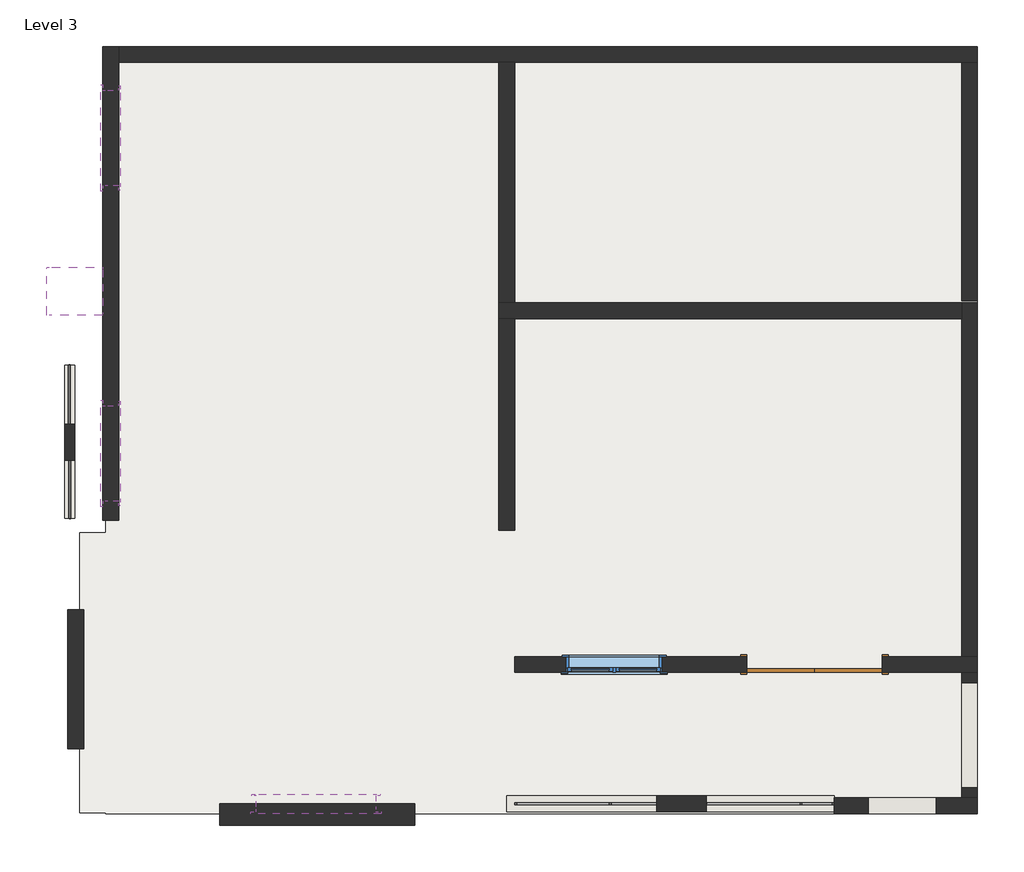
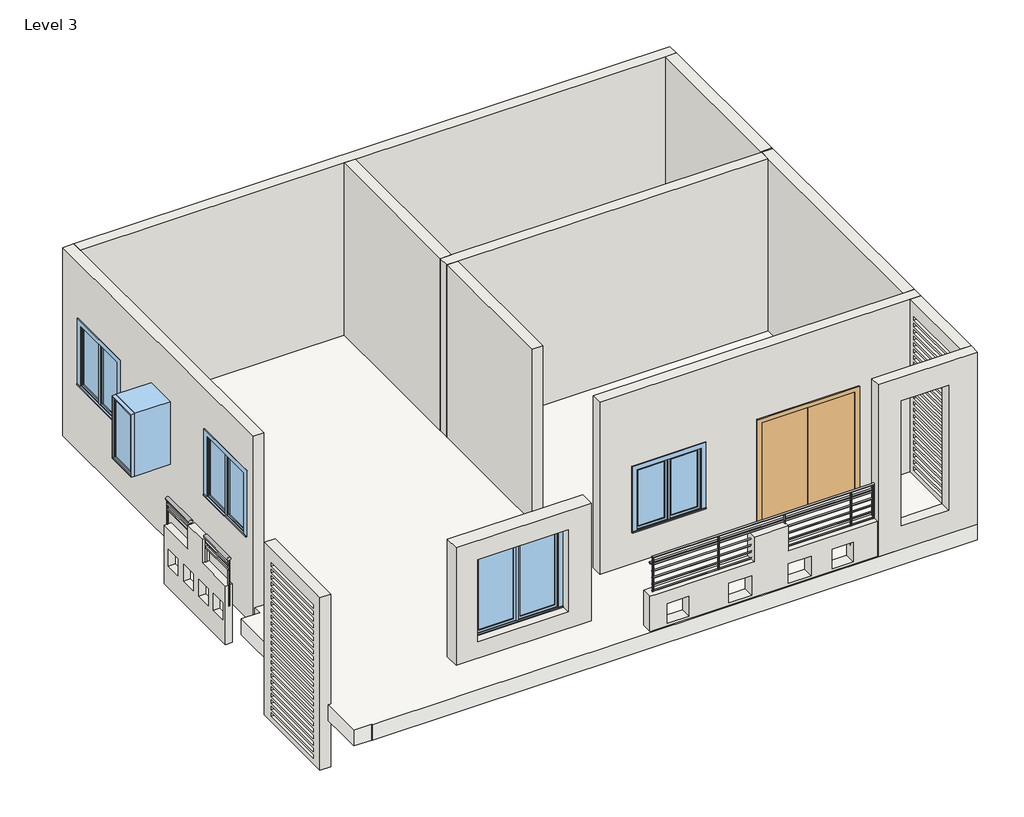
# One storey: 14 walls, 5 windows, 3 railings, 1 door, 1 roof.
"""IFC4 building model written with IfcOpenShell, lengths in millimetres."""

from ifc_helpers import new_model, si_unit, point, frame, frame_2d, origin, place, context, project, spatial, polyline, circle_curve, ellipse_curve, trimmed, segment, composite_curve, outline, extrude, faceted_brep, transform, mapped, element, save
from ifc_brep_helpers import plane_surface, extruded_surface, advanced_brep
from components import door_aae36eb6, walls_3_walls_1_8b7cdd2a, window_0862ab64, window_514a67b1, window_df4b05bc

model = new_model("IFC4")

# Units and contexts
model_context = context("Model", 3, world=origin())
ifc_project = project(units=[si_unit("LENGTHUNIT", "METRE", prefix="MILLI")], contexts=[model_context])

# Site, building, storey
site = spatial("IfcSite", under=ifc_project)
building = spatial("IfcBuilding", under=site)
storey = spatial("IfcBuildingStorey", under=building, Name="Level 3", Elevation=7315.2)

# Door
placement = place(None, origin())
door_shape = door_aae36eb6(model_context)
element("IfcDoor", 1, ObjectType="Door-Double-Flush_Panel : 68\" x 80\"", at=placement, inside=storey, context=model_context, shape_type="MappedRepresentation", body=[
    mapped(door_shape, transform((-960.1997472, 3460.2484482, 7518.4), x_axis=(-1.0, 0.0, 0.0), y_axis=(0.0, -1.0, 0.0), z_axis=(0.0, 0.0, 1.0))),
])

# Railings
element("IfcRailing", 2, ObjectType="Glass Panel - Bottom Fill", at=placement, inside=storey, context=model_context, shape_type="SolidModel", body=[
    advanced_brep(
    [(-10443.9247472, 7286.192958, 8717.2601563), (-10520.1247472, 7286.192958, 8717.2601563), (-10443.9247472, 6531.4144874, 8717.2601563), (-10520.1247472, 6531.4144874, 8717.2601563)],
    [
        (0, 1, ellipse_curve(frame((-10482.0247472, 7286.192958, 8717.2601563), z_axis=(0.0, 1.0, 0.0), x_axis=(-1.0, 0.0, 0.0)), 38.1, 28.575)),
        (1, 0, ellipse_curve(frame((-10482.0247472, 7286.192958, 8717.2601563), z_axis=(0.0, 1.0, 0.0), x_axis=(-1.0, 0.0, 0.0)), 38.1, 28.575)),
        (2, 3, ellipse_curve(frame((-10482.0247472, 6531.4144874, 8717.2601563), z_axis=(0.0, -1.0, 0.0), x_axis=(-1.0, 0.0, 0.0)), 38.1, 28.575)),
        (3, 2, ellipse_curve(frame((-10482.0247472, 6531.4144874, 8717.2601563), z_axis=(0.0, -1.0, 0.0), x_axis=(-1.0, 0.0, 0.0)), 38.1, 28.575)),
        (0, 2),
        (3, 1),
    ],
    [
        plane_surface(frame((-10482.0247472, 7286.192958, 8717.2601563), z_axis=(0.0, 1.0, 0.0), x_axis=(0.0, 0.0, -1.0))),
        plane_surface(frame((-10482.0247472, 6531.4144874, 8717.2601563), z_axis=(0.0, -1.0, 0.0), x_axis=(0.0, 0.0, -1.0))),
        extruded_surface(trimmed(ellipse_curve(frame((-10482.0247472, 6531.4144874, 8717.2601563), z_axis=(0.0, 1.0, 0.0), x_axis=(-1.0, 0.0, 0.0)), 38.1, 28.575), [point((-10443.9247472, 6531.4144874, 8717.2601563))], [point((-10520.1247472, 6531.4144874, 8717.2601563))], True, "CARTESIAN"), (0.0, 754.7784705999993, 0.0), 754.7784705999993),
        extruded_surface(trimmed(ellipse_curve(frame((-10482.0247472, 6531.4144874, 8717.2601563), z_axis=(0.0, 1.0, 0.0), x_axis=(-1.0, 0.0, 0.0)), 38.1, 28.575), [point((-10520.1247472, 6531.4144874, 8717.2601563))], [point((-10443.9247472, 6531.4144874, 8717.2601563))], True, "CARTESIAN"), (0.0, 754.7784705999993, 0.0), 754.7784705999993),
    ],
    [
        (0, [[1, 2]]),
        (1, [[3, 4]]),
        (2, [[-1, 5, -4, 6]]),
        (3, [[-2, -6, -3, -5]]),
    ],
),
    extrude(outline(polyline([(-10494.7247472, 7286.192958), (-10469.3247472, 7286.192958), (-10469.3247472, 6531.4144874), (-10494.7247472, 6531.4144874), (-10494.7247472, 7286.192958)])), frame((0.0, 0.0, 8602.9601563), z_axis=(0.0, 0.0, 1.0), x_axis=(1.0, 0.0, 0.0)), (0.0, 0.0, 1.0), 25.4),
    extrude(outline(polyline([(-10494.7247472, 7286.192958), (-10469.3247472, 7286.192958), (-10469.3247472, 6531.4144874), (-10494.7247472, 6531.4144874), (-10494.7247472, 7286.192958)])), frame((0.0, 0.0, 8501.3601563), z_axis=(0.0, 0.0, 1.0), x_axis=(1.0, 0.0, 0.0)), (0.0, 0.0, 1.0), 25.4),
    extrude(outline(polyline([(-10491.5497472, 6544.1144874), (-10472.4997472, 6544.1144874), (-10472.4997472, 6525.0644874), (-10491.5497472, 6525.0644874), (-10491.5497472, 6544.1144874)])), frame((0.0, 0.0, 7802.8601563), z_axis=(0.0, 0.0, 1.0), x_axis=(1.0, 0.0, 0.0)), (0.0, 0.0, 1.0), 885.6788223),
    extrude(outline(polyline([(-10491.5497472, 7292.542958), (-10472.4997472, 7292.542958), (-10472.4997472, 7273.492958), (-10491.5497472, 7273.492958), (-10491.5497472, 7292.542958)])), frame((0.0, 0.0, 7802.8601563), z_axis=(0.0, 0.0, 1.0), x_axis=(1.0, 0.0, 0.0)), (0.0, 0.0, 1.0), 885.6788223),
])
element("IfcRailing", 3, ObjectType="Glass Panel - Bottom Fill", at=placement, inside=storey, context=model_context, shape_type="SolidModel", body=[
    advanced_brep(
    [(-10437.5747472, 6074.2144874, 8717.2601563), (-10513.7747472, 6074.2144874, 8717.2601563), (-10437.5747472, 5330.392958, 8717.2601563), (-10513.7747472, 5330.392958, 8717.2601563)],
    [
        (0, 1, ellipse_curve(frame((-10475.6747472, 6074.2144874, 8717.2601563), z_axis=(0.0, 1.0, 0.0), x_axis=(-1.0, 0.0, 0.0)), 38.1, 28.575)),
        (1, 0, ellipse_curve(frame((-10475.6747472, 6074.2144874, 8717.2601563), z_axis=(0.0, 1.0, 0.0), x_axis=(-1.0, 0.0, 0.0)), 38.1, 28.575)),
        (2, 3, ellipse_curve(frame((-10475.6747472, 5330.392958, 8717.2601563), z_axis=(0.0, -1.0, 0.0), x_axis=(-1.0, 0.0, 0.0)), 38.1, 28.575)),
        (3, 2, ellipse_curve(frame((-10475.6747472, 5330.392958, 8717.2601563), z_axis=(0.0, -1.0, 0.0), x_axis=(-1.0, 0.0, 0.0)), 38.1, 28.575)),
        (0, 2),
        (3, 1),
    ],
    [
        plane_surface(frame((-10475.6747472, 6074.2144874, 8717.2601563), z_axis=(0.0, 1.0, 0.0), x_axis=(0.0, 0.0, -1.0))),
        plane_surface(frame((-10475.6747472, 5330.392958, 8717.2601563), z_axis=(0.0, -1.0, 0.0), x_axis=(0.0, 0.0, -1.0))),
        extruded_surface(trimmed(ellipse_curve(frame((-10475.6747472, 5330.392958, 8717.2601563), z_axis=(0.0, 1.0, 0.0), x_axis=(-1.0, 0.0, 0.0)), 38.1, 28.575), [point((-10437.5747472, 5330.392958, 8717.2601563))], [point((-10513.7747472, 5330.392958, 8717.2601563))], True, "CARTESIAN"), (0.0, 743.8215293999992, 0.0), 743.8215293999992),
        extruded_surface(trimmed(ellipse_curve(frame((-10475.6747472, 5330.392958, 8717.2601563), z_axis=(0.0, 1.0, 0.0), x_axis=(-1.0, 0.0, 0.0)), 38.1, 28.575), [point((-10513.7747472, 5330.392958, 8717.2601563))], [point((-10437.5747472, 5330.392958, 8717.2601563))], True, "CARTESIAN"), (0.0, 743.8215293999992, 0.0), 743.8215293999992),
    ],
    [
        (0, [[1, 2]]),
        (1, [[3, 4]]),
        (2, [[-1, 5, -4, 6]]),
        (3, [[-2, -6, -3, -5]]),
    ],
),
    extrude(outline(polyline([(-10488.3747472, 6074.2144874), (-10462.9747472, 6074.2144874), (-10462.9747472, 5330.392958), (-10488.3747472, 5330.392958), (-10488.3747472, 6074.2144874)])), frame((0.0, 0.0, 8602.9601563), z_axis=(0.0, 0.0, 1.0), x_axis=(1.0, 0.0, 0.0)), (0.0, 0.0, 1.0), 25.4),
    extrude(outline(polyline([(-10488.3747472, 6074.2144874), (-10462.9747472, 6074.2144874), (-10462.9747472, 5330.392958), (-10488.3747472, 5330.392958), (-10488.3747472, 6074.2144874)])), frame((0.0, 0.0, 8501.3601563), z_axis=(0.0, 0.0, 1.0), x_axis=(1.0, 0.0, 0.0)), (0.0, 0.0, 1.0), 25.4),
    extrude(outline(polyline([(-10485.1997472, 5343.092958), (-10466.1497472, 5343.092958), (-10466.1497472, 5324.042958), (-10485.1997472, 5324.042958), (-10485.1997472, 5343.092958)])), frame((0.0, 0.0, 7802.8601563), z_axis=(0.0, 0.0, 1.0), x_axis=(1.0, 0.0, 0.0)), (0.0, 0.0, 1.0), 885.6788223),
    extrude(outline(polyline([(-10485.1997472, 6080.5644874), (-10466.1497472, 6080.5644874), (-10466.1497472, 6061.5144874), (-10485.1997472, 6061.5144874), (-10485.1997472, 6080.5644874)])), frame((0.0, 0.0, 7802.8601563), z_axis=(0.0, 0.0, 1.0), x_axis=(1.0, 0.0, 0.0)), (0.0, 0.0, 1.0), 885.6788223),
])
element("IfcRailing", 4, ObjectType="Guardrail - Pipe", at=placement, inside=storey, context=model_context, shape_type="SweptSolid", body=[
    extrude(outline(composite_curve([segment(trimmed(circle_curve(frame_2d((1758.4484482, 8820.15)), 19.05), [point((1739.3984482, 8820.15))], [point((1777.4984482, 8820.15))], False, "CARTESIAN"), True, "CONTINUOUS"), segment(trimmed(circle_curve(frame_2d((1758.4484482, 8820.15)), 19.05), [point((1777.4984482, 8820.15))], [point((1739.3984482, 8820.15))], False, "CARTESIAN"), True, "CONTINUOUS")], self_intersect=False)), frame((-4789.9857575, 0.0, 0.0), z_axis=(1.0, 0.0, 0.0), x_axis=(0.0, 1.0, 0.0)), (0.0, 0.0, 1.0), 4083.7860103),
    extrude(outline(composite_curve([segment(trimmed(circle_curve(frame_2d((1682.2484482, 8972.55)), 19.05), [point((1663.1984482, 8972.55))], [point((1701.2984482, 8972.55))], False, "CARTESIAN"), True, "CONTINUOUS"), segment(trimmed(circle_curve(frame_2d((1682.2484482, 8972.55)), 19.05), [point((1701.2984482, 8972.55))], [point((1663.1984482, 8972.55))], False, "CARTESIAN"), True, "CONTINUOUS")], self_intersect=False)), frame((-4789.9857575, 0.0, 0.0), z_axis=(1.0, 0.0, 0.0), x_axis=(0.0, 1.0, 0.0)), (0.0, 0.0, 1.0), 4083.7860103),
    extrude(outline(composite_curve([segment(trimmed(circle_curve(frame_2d((1682.2484482, 8826.5)), 12.7), [point((1694.9484482, 8826.5))], [point((1669.5484482, 8826.5))], False, "CARTESIAN"), True, "CONTINUOUS"), segment(trimmed(circle_curve(frame_2d((1682.2484482, 8826.5)), 12.7), [point((1669.5484482, 8826.5))], [point((1694.9484482, 8826.5))], False, "CARTESIAN"), True, "CONTINUOUS")], self_intersect=False)), frame((-4789.9857575, 0.0, 0.0), z_axis=(1.0, 0.0, 0.0), x_axis=(0.0, 1.0, 0.0)), (0.0, 0.0, 1.0), 4083.7860103),
    extrude(outline(composite_curve([segment(trimmed(circle_curve(frame_2d((1682.2484482, 8699.5)), 12.7), [point((1694.9484482, 8699.5))], [point((1669.5484482, 8699.5))], False, "CARTESIAN"), True, "CONTINUOUS"), segment(trimmed(circle_curve(frame_2d((1682.2484482, 8699.5)), 12.7), [point((1669.5484482, 8699.5))], [point((1694.9484482, 8699.5))], False, "CARTESIAN"), True, "CONTINUOUS")], self_intersect=False)), frame((-4789.9857575, 0.0, 0.0), z_axis=(1.0, 0.0, 0.0), x_axis=(0.0, 1.0, 0.0)), (0.0, 0.0, 1.0), 4083.7860103),
    extrude(outline(composite_curve([segment(trimmed(circle_curve(frame_2d((1682.2484482, 8572.5)), 12.7), [point((1694.9484482, 8572.5))], [point((1669.5484482, 8572.5))], False, "CARTESIAN"), True, "CONTINUOUS"), segment(trimmed(circle_curve(frame_2d((1682.2484482, 8572.5)), 12.7), [point((1669.5484482, 8572.5))], [point((1694.9484482, 8572.5))], False, "CARTESIAN"), True, "CONTINUOUS")], self_intersect=False)), frame((-4789.9857575, 0.0, 0.0), z_axis=(1.0, 0.0, 0.0), x_axis=(0.0, 1.0, 0.0)), (0.0, 0.0, 1.0), 4083.7860103),
    extrude(outline(composite_curve([segment(trimmed(circle_curve(frame_2d((1682.2484482, 8445.5)), 12.7), [point((1694.9484482, 8445.5))], [point((1669.5484482, 8445.5))], False, "CARTESIAN"), True, "CONTINUOUS"), segment(trimmed(circle_curve(frame_2d((1682.2484482, 8445.5)), 12.7), [point((1669.5484482, 8445.5))], [point((1694.9484482, 8445.5))], False, "CARTESIAN"), True, "CONTINUOUS")], self_intersect=False)), frame((-4789.9857575, 0.0, 0.0), z_axis=(1.0, 0.0, 0.0), x_axis=(0.0, 1.0, 0.0)), (0.0, 0.0, 1.0), 4083.7860103),
    extrude(outline(composite_curve([segment(trimmed(circle_curve(frame_2d((1682.2484482, 8318.5)), 12.7), [point((1694.9484482, 8318.5))], [point((1669.5484482, 8318.5))], False, "CARTESIAN"), True, "CONTINUOUS"), segment(trimmed(circle_curve(frame_2d((1682.2484482, 8318.5)), 12.7), [point((1669.5484482, 8318.5))], [point((1694.9484482, 8318.5))], False, "CARTESIAN"), True, "CONTINUOUS")], self_intersect=False)), frame((-4789.9857575, 0.0, 0.0), z_axis=(1.0, 0.0, 0.0), x_axis=(0.0, 1.0, 0.0)), (0.0, 0.0, 1.0), 4083.7860103),
    extrude(outline(composite_curve([segment(trimmed(circle_curve(frame_2d((1682.2484482, 8191.5)), 12.7), [point((1694.9484482, 8191.5))], [point((1669.5484482, 8191.5))], False, "CARTESIAN"), True, "CONTINUOUS"), segment(trimmed(circle_curve(frame_2d((1682.2484482, 8191.5)), 12.7), [point((1669.5484482, 8191.5))], [point((1694.9484482, 8191.5))], False, "CARTESIAN"), True, "CONTINUOUS")], self_intersect=False)), frame((-4789.9857575, 0.0, 0.0), z_axis=(1.0, 0.0, 0.0), x_axis=(0.0, 1.0, 0.0)), (0.0, 0.0, 1.0), 4083.7860103),
    extrude(outline(composite_curve([segment(trimmed(circle_curve(frame_2d((1682.2484482, 8064.5)), 12.7), [point((1694.9484482, 8064.5))], [point((1669.5484482, 8064.5))], False, "CARTESIAN"), True, "CONTINUOUS"), segment(trimmed(circle_curve(frame_2d((1682.2484482, 8064.5)), 12.7), [point((1669.5484482, 8064.5))], [point((1694.9484482, 8064.5))], False, "CARTESIAN"), True, "CONTINUOUS")], self_intersect=False)), frame((-4789.9857575, 0.0, 0.0), z_axis=(1.0, 0.0, 0.0), x_axis=(0.0, 1.0, 0.0)), (0.0, 0.0, 1.0), 4083.7860103),
    extrude(outline(composite_curve([segment(trimmed(circle_curve(frame_2d((-1132.3857575, 1682.2484482)), 12.7), [point((-1132.3857575, 1694.9484482))], [point((-1132.3857575, 1669.5484482))], False, "CARTESIAN"), True, "CONTINUOUS"), segment(trimmed(circle_curve(frame_2d((-1132.3857575, 1682.2484482)), 12.7), [point((-1132.3857575, 1669.5484482))], [point((-1132.3857575, 1694.9484482))], False, "CARTESIAN"), True, "CONTINUOUS")], self_intersect=False)), frame((0.0, 0.0, 7924.8), z_axis=(0.0, 0.0, 1.0), x_axis=(1.0, 0.0, 0.0)), (0.0, 0.0, 1.0), 1028.7),
    extrude(outline(composite_curve([segment(trimmed(circle_curve(frame_2d((-2351.5857575, 1682.2484482)), 12.7), [point((-2351.5857575, 1694.9484482))], [point((-2351.5857575, 1669.5484482))], False, "CARTESIAN"), True, "CONTINUOUS"), segment(trimmed(circle_curve(frame_2d((-2351.5857575, 1682.2484482)), 12.7), [point((-2351.5857575, 1669.5484482))], [point((-2351.5857575, 1694.9484482))], False, "CARTESIAN"), True, "CONTINUOUS")], self_intersect=False)), frame((0.0, 0.0, 7924.8), z_axis=(0.0, 0.0, 1.0), x_axis=(1.0, 0.0, 0.0)), (0.0, 0.0, 1.0), 1028.7),
    extrude(outline(composite_curve([segment(trimmed(circle_curve(frame_2d((-3570.7857575, 1682.2484482)), 12.7), [point((-3570.7857575, 1694.9484482))], [point((-3570.7857575, 1669.5484482))], False, "CARTESIAN"), True, "CONTINUOUS"), segment(trimmed(circle_curve(frame_2d((-3570.7857575, 1682.2484482)), 12.7), [point((-3570.7857575, 1669.5484482))], [point((-3570.7857575, 1694.9484482))], False, "CARTESIAN"), True, "CONTINUOUS")], self_intersect=False)), frame((0.0, 0.0, 7924.8), z_axis=(0.0, 0.0, 1.0), x_axis=(1.0, 0.0, 0.0)), (0.0, 0.0, 1.0), 1028.7),
    extrude(outline(composite_curve([segment(trimmed(circle_curve(frame_2d((-718.8997472, 1682.2484482)), 12.7), [point((-718.8997472, 1694.9484482))], [point((-718.8997472, 1669.5484482))], False, "CARTESIAN"), True, "CONTINUOUS"), segment(trimmed(circle_curve(frame_2d((-718.8997472, 1682.2484482)), 12.7), [point((-718.8997472, 1669.5484482))], [point((-718.8997472, 1694.9484482))], False, "CARTESIAN"), True, "CONTINUOUS")], self_intersect=False)), frame((0.0, 0.0, 7924.8), z_axis=(0.0, 0.0, 1.0), x_axis=(1.0, 0.0, 0.0)), (0.0, 0.0, 1.0), 1028.7),
    extrude(outline(composite_curve([segment(trimmed(circle_curve(frame_2d((-4777.2857575, 1682.2484482)), 12.7), [point((-4777.2857575, 1694.9484482))], [point((-4777.2857575, 1669.5484482))], False, "CARTESIAN"), True, "CONTINUOUS"), segment(trimmed(circle_curve(frame_2d((-4777.2857575, 1682.2484482)), 12.7), [point((-4777.2857575, 1669.5484482))], [point((-4777.2857575, 1694.9484482))], False, "CARTESIAN"), True, "CONTINUOUS")], self_intersect=False)), frame((0.0, 0.0, 7924.8), z_axis=(0.0, 0.0, 1.0), x_axis=(1.0, 0.0, 0.0)), (0.0, 0.0, 1.0), 1028.7),
])

# Roof
element("IfcRoof", 5, ObjectType="Generic - 12\"", at=placement, inside=storey, context=model_context, shape_type="SweptSolid", body=[
    extrude(outline(polyline([(-10018.4747472, 11358.0609482), (1122.6002528, 11358.0609482), (1122.6002528, 1553.6609482), (-10019.8638097, 1553.6609482), (-10019.8638097, 1567.9484482), (-10352.5857575, 1567.9484482), (-10352.5857575, 5144.9959854), (-10018.4747472, 5144.9959854), (-10018.4747472, 11358.0609482)])), frame((0.0, 0.0, 7315.2), z_axis=(0.0, 0.0, 1.0), x_axis=(1.0, 0.0, 0.0)), (0.0, 0.0, 1.0), 304.8),
])

# Walls
element("IfcWall", 6, ObjectType="Generic - 5\"", at=placement, inside=storey, context=model_context, shape_type="SweptSolid", body=[
    extrude(outline(polyline([(7286.192958, 7071.0386364), (5330.392958, 7071.0386364), (5330.392958, 8212.2632192), (6074.2144874, 8212.2632192), (6074.2144874, 8669.4632192), (6531.4144874, 8669.4632192), (6531.4144874, 8212.2632192), (7286.192958, 8212.2632192), (7286.192958, 7071.0386364)]), holes=[polyline([(6843.8232349, 7827.9459623), (6843.8232349, 7497.7459623), (7148.6232349, 7497.7459623), (7148.6232349, 7827.9459623), (6843.8232349, 7827.9459623)]), polyline([(6361.2232349, 7827.9459623), (6361.2232349, 7497.7459623), (6666.0232349, 7497.7459623), (6666.0232349, 7827.9459623), (6361.2232349, 7827.9459623)]), polyline([(5878.6232349, 7827.9459623), (5878.6232349, 7497.7459623), (6183.4232349, 7497.7459623), (6183.4232349, 7827.9459623), (5878.6232349, 7827.9459623)]), polyline([(5421.4232349, 7827.9459623), (5421.4232349, 7497.7459623), (5726.2232349, 7497.7459623), (5726.2232349, 7827.9459623), (5421.4232349, 7827.9459623)])]), frame((-10539.1747472, 0.0, 0.0), z_axis=(1.0, 0.0, 0.0), x_axis=(0.0, 1.0, 0.0)), (0.0, 0.0, 1.0), 127.0),
])
element("IfcWall", 7, ObjectType="Generic - 8\"", at=placement, inside=storey, context=model_context, shape_type="Brep", body=[
    faceted_brep([(-4789.9857575, 3358.6484482, 7315.2), (1122.6002528, 3358.6484482, 7315.2), (1122.6002528, 3358.6484482, 7620.0), (1122.6002528, 3358.6484482, 10972.8), (-4789.9857575, 3358.6484482, 10972.8), (-1823.7997472, 3358.6484482, 7518.4), (-1823.7997472, 3358.6484482, 9550.4), (-96.5997472, 3358.6484482, 9550.4), (-96.5997472, 3358.6484482, 7518.4), (-4129.5857575, 3358.6484482, 8229.6), (-4129.5857575, 3358.6484482, 9448.8), (-2910.3857575, 3358.6484482, 9448.8), (-2910.3857575, 3358.6484482, 8229.6), (1122.6002528, 3561.8484482, 7315.2), (919.4002528, 3561.8484482, 7315.2), (-4789.9857575, 3561.8484482, 7315.2), (-4789.9857575, 3561.8484482, 10972.8), (919.4002528, 3561.8484482, 10972.8), (1122.6002528, 3561.8484482, 10972.8), (-1823.7997472, 3561.8484482, 9550.4), (-1823.7997472, 3561.8484482, 7518.4), (-96.5997472, 3561.8484482, 7518.4), (-96.5997472, 3561.8484482, 9550.4), (-4129.5857575, 3561.8484482, 9448.8), (-4129.5857575, 3561.8484482, 8229.6), (-2910.3857575, 3561.8484482, 8229.6), (-2910.3857575, 3561.8484482, 9448.8)], [[[0, 1, 2, 3, 4], [5, 6, 7, 8], [9, 10, 11, 12]], [[13, 14, 15, 16, 17, 18], [19, 20, 21, 22], [23, 24, 25, 26]], [[1, 0, 15, 14, 13]], [[4, 3, 18, 17, 16]], [[0, 4, 16, 15]], [[1, 13, 18, 3, 2]], [[5, 20, 19, 6]], [[6, 19, 22, 7]], [[7, 22, 21, 8]], [[20, 5, 8, 21]], [[24, 23, 10, 9]], [[25, 24, 9, 12]], [[26, 25, 12, 11]], [[23, 26, 11, 10]]]),
])
element("IfcWall", 8, ObjectType="Generic - 8\"", at=placement, inside=storey, context=model_context, shape_type="Brep", body=[
    faceted_brep([(1122.6002528, 3561.8484482, 10972.8), (1122.6002528, 3561.8484482, 7315.2), (1122.6002528, 8083.0484482, 7315.2), (1122.6002528, 8083.0484482, 10972.8), (919.4002528, 3561.8484482, 7315.2), (919.4002528, 3561.8484482, 10972.8), (919.4002528, 7879.8484482, 10972.8), (919.4002528, 8083.0484482, 10972.8), (919.4002528, 8083.0484482, 7315.2), (919.4002528, 7879.8484482, 7315.2)], [[[0, 1, 2, 3]], [[4, 5, 6, 7, 8, 9]], [[2, 1, 4, 9, 8]], [[0, 3, 7, 6, 5]], [[3, 2, 8, 7]], [[0, 5, 4, 1]]]),
])
element("IfcWall", 9, ObjectType="Generic - 8\"", at=placement, inside=storey, context=model_context, shape_type="Brep", body=[
    faceted_brep([(919.4002528, 8083.0484482, 7315.2), (-4789.9857575, 8083.0484482, 7315.2), (-4993.1857575, 8083.0484482, 7315.2), (-4993.1857575, 8083.0484482, 10972.8), (-4789.9857575, 8083.0484482, 10972.8), (919.4002528, 8083.0484482, 10972.8), (919.4002528, 7879.8484482, 7315.2), (919.4002528, 7879.8484482, 10972.8), (-4789.9857575, 7879.8484482, 10972.8), (-4993.1857575, 7879.8484482, 10972.8), (-4993.1857575, 7879.8484482, 7315.2), (-4789.9857575, 7879.8484482, 7315.2)], [[[0, 1, 2, 3, 4, 5]], [[6, 7, 8, 9, 10, 11]], [[2, 1, 0, 6, 11, 10]], [[5, 4, 3, 9, 8, 7]], [[0, 5, 7, 6]], [[3, 2, 10, 9]]]),
])
element("IfcWall", 10, ObjectType="Generic - 8\"", at=placement, inside=storey, context=model_context, shape_type="SweptSolid", body=[
    extrude(outline(polyline([(-4993.1857575, 5174.7484482), (-4993.1857575, 7879.8484482), (-4789.9857575, 7879.8484482), (-4789.9857575, 5174.7484482), (-4993.1857575, 5174.7484482)])), frame((0.0, 0.0, 7315.2), z_axis=(0.0, 0.0, 1.0), x_axis=(1.0, 0.0, 0.0)), (0.0, 0.0, 1.0), 3657.6),
])
element("IfcWall", 11, ObjectType="Generic - 8\"", at=placement, inside=storey, context=model_context, shape_type="Brep", body=[
    faceted_brep([(-9850.1997472, 5306.9209854, 7315.2), (-9850.1997472, 11154.8609482, 7315.2), (-9850.1997472, 11358.0609482, 7315.2), (-9850.1997472, 11358.0609482, 10972.8), (-9850.1997472, 11154.8609482, 10972.8), (-9850.1997472, 5306.9209854, 10972.8), (-9850.1997472, 6767.4209854, 10126.4336549), (-9850.1997472, 6767.4209854, 8907.2336549), (-9850.1997472, 5548.2209854, 8907.2336549), (-9850.1997472, 5548.2209854, 10126.4336549), (-9850.1997472, 10799.2609482, 9827.5564612), (-9850.1997472, 10799.2609482, 8608.3564612), (-9850.1997472, 9580.0609482, 8608.3564612), (-9850.1997472, 9580.0609482, 9827.5564612), (-10053.3997472, 5306.9209854, 7315.2), (-10053.3997472, 5306.9209854, 10972.8), (-10053.3997472, 11358.0609482, 10972.8), (-10053.3997472, 11358.0609482, 7315.2), (-10053.3997472, 6767.4209854, 10126.4336549), (-10053.3997472, 5548.2209854, 10126.4336549), (-10053.3997472, 5548.2209854, 8907.2336549), (-10053.3997472, 6767.4209854, 8907.2336549), (-10053.3997472, 10799.2609482, 9827.5564612), (-10053.3997472, 9580.0609482, 9827.5564612), (-10053.3997472, 9580.0609482, 8608.3564612), (-10053.3997472, 10799.2609482, 8608.3564612)], [[[0, 1, 2, 3, 4, 5], [6, 7, 8, 9], [10, 11, 12, 13]], [[14, 15, 16, 17], [18, 19, 20, 21], [22, 23, 24, 25]], [[2, 1, 0, 14, 17]], [[5, 4, 3, 16, 15]], [[3, 2, 17, 16]], [[0, 5, 15, 14]], [[7, 6, 18, 21]], [[8, 7, 21, 20]], [[9, 8, 20, 19]], [[6, 9, 19, 18]], [[11, 10, 22, 25]], [[12, 11, 25, 24]], [[13, 12, 24, 23]], [[10, 13, 23, 22]]]),
])
element("IfcWall", 12, ObjectType="Generic - 8\"", at=placement, inside=storey, context=model_context, shape_type="Brep", body=[
    faceted_brep([(-9850.1997472, 11154.8609482, 7315.2), (-4993.1857575, 11154.8609482, 7315.2), (-4789.9857575, 11154.8609482, 7315.2), (919.4002528, 11154.8609482, 7315.2), (1122.6002528, 11154.8609482, 7315.2), (1122.6002528, 11154.8609482, 10972.8), (919.4002528, 11154.8609482, 10972.8), (-4789.9857575, 11154.8609482, 10972.8), (-4993.1857575, 11154.8609482, 10972.8), (-9850.1997472, 11154.8609482, 10972.8), (-9850.1997472, 11358.0609482, 7315.2), (-9850.1997472, 11358.0609482, 10972.8), (1122.6002528, 11358.0609482, 10972.8), (1122.6002528, 11358.0609482, 7315.2)], [[[0, 1, 2, 3, 4, 5, 6, 7, 8, 9]], [[10, 11, 12, 13]], [[4, 3, 2, 1, 0, 10, 13]], [[9, 8, 7, 6, 5, 12, 11]], [[0, 9, 11, 10]], [[5, 4, 13, 12]]]),
])
element("IfcWall", 13, ObjectType="Generic - 8\"", at=placement, inside=storey, context=model_context, shape_type="SweptSolid", body=[
    extrude(outline(polyline([(919.4002528, 8106.8609482), (919.4002528, 11154.8609482), (1122.6002528, 11154.8609482), (1122.6002528, 8106.8609482), (919.4002528, 8106.8609482)])), frame((0.0, 0.0, 7315.2), z_axis=(0.0, 0.0, 1.0), x_axis=(1.0, 0.0, 0.0)), (0.0, 0.0, 1.0), 3657.6),
])
element("IfcWall", 14, ObjectType="Generic - 8\"", at=placement, inside=storey, context=model_context, shape_type="SweptSolid", body=[
    extrude(outline(polyline([(-4789.9857575, 11154.8609482), (-4789.9857575, 8083.0484482), (-4993.1857575, 8083.0484482), (-4993.1857575, 11154.8609482), (-4789.9857575, 11154.8609482)])), frame((0.0, 0.0, 7315.2), z_axis=(0.0, 0.0, 1.0), x_axis=(1.0, 0.0, 0.0)), (0.0, 0.0, 1.0), 3657.6),
])
element("IfcWall", 15, ObjectType="Generic - 8\"", at=placement, inside=storey, context=model_context, shape_type="SweptSolid", body=[
    extrude(outline(polyline([(7626.4207699, 1122.6002528), (10972.8, 1122.6002528), (10972.8, -706.1997472), (7626.4207699, -706.1997472), (7626.4207699, 1122.6002528)]), holes=[polyline([(10516.412956, 593.7729517), (8078.012956, 593.7729517), (8078.012956, -276.1770483), (10516.412956, -276.1770483), (10516.412956, 593.7729517)])]), frame((0.0, 1553.6609482, 0.0), z_axis=(0.0, 1.0, 0.0), x_axis=(0.0, 0.0, 1.0)), (0.0, 0.0, 1.0), 203.2),
])
element("IfcWall", 16, ObjectType="Generic - 8\"", at=placement, inside=storey, context=model_context, shape_type="Brep", body=[
    faceted_brep([(1122.6002528, 3358.6484482, 7620.0), (1122.6002528, 3358.6484482, 10972.8), (1122.6002528, 1756.8609482, 10972.8), (1122.6002528, 1756.8609482, 7626.4207699), (1122.6002528, 1756.8609482, 7620.0), (1122.6002528, 3228.8895121, 10714.2542182), (1122.6002528, 3228.8895121, 10650.7542182), (1122.6002528, 1882.6895121, 10650.7542182), (1122.6002528, 1882.6895121, 10714.2542182), (1122.6002528, 3228.8895121, 10587.2542182), (1122.6002528, 3228.8895121, 10523.7542182), (1122.6002528, 1882.6895121, 10523.7542182), (1122.6002528, 1882.6895121, 10587.2542182), (1122.6002528, 3228.8895121, 10460.2542182), (1122.6002528, 3228.8895121, 10396.7542182), (1122.6002528, 1882.6895121, 10396.7542182), (1122.6002528, 1882.6895121, 10460.2542182), (1122.6002528, 3228.8895121, 10333.2542182), (1122.6002528, 3228.8895121, 10269.7542182), (1122.6002528, 1882.6895121, 10269.7542182), (1122.6002528, 1882.6895121, 10333.2542182), (1122.6002528, 3228.8895121, 10206.2542182), (1122.6002528, 3228.8895121, 10142.7542182), (1122.6002528, 1882.6895121, 10142.7542182), (1122.6002528, 1882.6895121, 10206.2542182), (1122.6002528, 3228.8895121, 10079.2542182), (1122.6002528, 3228.8895121, 10015.7542182), (1122.6002528, 1882.6895121, 10015.7542182), (1122.6002528, 1882.6895121, 10079.2542182), (1122.6002528, 3228.8895121, 9952.2542182), (1122.6002528, 3228.8895121, 9888.7542182), (1122.6002528, 1882.6895121, 9888.7542182), (1122.6002528, 1882.6895121, 9952.2542182), (1122.6002528, 3228.8895121, 9825.2542182), (1122.6002528, 3228.8895121, 9761.7542182), (1122.6002528, 1882.6895121, 9761.7542182), (1122.6002528, 1882.6895121, 9825.2542182), (1122.6002528, 3228.8895121, 9698.2542182), (1122.6002528, 3228.8895121, 9634.7542182), (1122.6002528, 1882.6895121, 9634.7542182), (1122.6002528, 1882.6895121, 9698.2542182), (1122.6002528, 3228.8895121, 9571.2542182), (1122.6002528, 3228.8895121, 9507.7542182), (1122.6002528, 1882.6895121, 9507.7542182), (1122.6002528, 1882.6895121, 9571.2542182), (1122.6002528, 3228.8895121, 9444.2542182), (1122.6002528, 3228.8895121, 9380.7542182), (1122.6002528, 1882.6895121, 9380.7542182), (1122.6002528, 1882.6895121, 9444.2542182), (1122.6002528, 3228.8895121, 9317.2542182), (1122.6002528, 3228.8895121, 9253.7542182), (1122.6002528, 1882.6895121, 9253.7542182), (1122.6002528, 1882.6895121, 9317.2542182), (1122.6002528, 3228.8895121, 9190.2542182), (1122.6002528, 3228.8895121, 9126.7542182), (1122.6002528, 1882.6895121, 9126.7542182), (1122.6002528, 1882.6895121, 9190.2542182), (1122.6002528, 3228.8895121, 9063.2542182), (1122.6002528, 3228.8895121, 8999.7542182), (1122.6002528, 1882.6895121, 8999.7542182), (1122.6002528, 1882.6895121, 9063.2542182), (1122.6002528, 3228.8895121, 8936.2542182), (1122.6002528, 3228.8895121, 8872.7542182), (1122.6002528, 1882.6895121, 8872.7542182), (1122.6002528, 1882.6895121, 8936.2542182), (1122.6002528, 3228.8895121, 8809.2542182), (1122.6002528, 3228.8895121, 8745.7542182), (1122.6002528, 1882.6895121, 8745.7542182), (1122.6002528, 1882.6895121, 8809.2542182), (1122.6002528, 3228.8895121, 8682.2542182), (1122.6002528, 3228.8895121, 8618.7542182), (1122.6002528, 1882.6895121, 8618.7542182), (1122.6002528, 1882.6895121, 8682.2542182), (1122.6002528, 3228.8895121, 8555.2542182), (1122.6002528, 3228.8895121, 8491.7542182), (1122.6002528, 1882.6895121, 8491.7542182), (1122.6002528, 1882.6895121, 8555.2542182), (1122.6002528, 3228.8895121, 8428.2542182), (1122.6002528, 3228.8895121, 8364.7542182), (1122.6002528, 1882.6895121, 8364.7542182), (1122.6002528, 1882.6895121, 8428.2542182), (1122.6002528, 3228.8895121, 8301.2542182), (1122.6002528, 3228.8895121, 8237.7542182), (1122.6002528, 1882.6895121, 8237.7542182), (1122.6002528, 1882.6895121, 8301.2542182), (1122.6002528, 3228.8895121, 8174.2542182), (1122.6002528, 3228.8895121, 8110.7542182), (1122.6002528, 1882.6895121, 8110.7542182), (1122.6002528, 1882.6895121, 8174.2542182), (1122.6002528, 3228.8895121, 8047.2542182), (1122.6002528, 3228.8895121, 7983.7542182), (1122.6002528, 1882.6895121, 7983.7542182), (1122.6002528, 1882.6895121, 8047.2542182), (1122.6002528, 3228.8895121, 7920.2542182), (1122.6002528, 3228.8895121, 7856.7542182), (1122.6002528, 1882.6895121, 7856.7542182), (1122.6002528, 1882.6895121, 7920.2542182), (1122.6002528, 3228.8895121, 7793.2542182), (1122.6002528, 3228.8895121, 7729.7542182), (1122.6002528, 1882.6895121, 7729.7542182), (1122.6002528, 1882.6895121, 7793.2542182), (919.4002528, 3358.6484482, 7620.0), (919.4002528, 1756.8609482, 7620.0), (919.4002528, 1756.8609482, 10972.8), (919.4002528, 3358.6484482, 10972.8), (919.4002528, 3228.8895121, 10714.2542182), (919.4002528, 1882.6895121, 10714.2542182), (919.4002528, 1882.6895121, 10650.7542182), (919.4002528, 3228.8895121, 10650.7542182), (919.4002528, 3228.8895121, 10587.2542182), (919.4002528, 1882.6895121, 10587.2542182), (919.4002528, 1882.6895121, 10523.7542182), (919.4002528, 3228.8895121, 10523.7542182), (919.4002528, 3228.8895121, 10460.2542182), (919.4002528, 1882.6895121, 10460.2542182), (919.4002528, 1882.6895121, 10396.7542182), (919.4002528, 3228.8895121, 10396.7542182), (919.4002528, 3228.8895121, 10333.2542182), (919.4002528, 1882.6895121, 10333.2542182), (919.4002528, 1882.6895121, 10269.7542182), (919.4002528, 3228.8895121, 10269.7542182), (919.4002528, 3228.8895121, 10206.2542182), (919.4002528, 1882.6895121, 10206.2542182), (919.4002528, 1882.6895121, 10142.7542182), (919.4002528, 3228.8895121, 10142.7542182), (919.4002528, 3228.8895121, 10079.2542182), (919.4002528, 1882.6895121, 10079.2542182), (919.4002528, 1882.6895121, 10015.7542182), (919.4002528, 3228.8895121, 10015.7542182), (919.4002528, 3228.8895121, 9952.2542182), (919.4002528, 1882.6895121, 9952.2542182), (919.4002528, 1882.6895121, 9888.7542182), (919.4002528, 3228.8895121, 9888.7542182), (919.4002528, 3228.8895121, 9825.2542182), (919.4002528, 1882.6895121, 9825.2542182), (919.4002528, 1882.6895121, 9761.7542182), (919.4002528, 3228.8895121, 9761.7542182), (919.4002528, 3228.8895121, 9698.2542182), (919.4002528, 1882.6895121, 9698.2542182), (919.4002528, 1882.6895121, 9634.7542182), (919.4002528, 3228.8895121, 9634.7542182), (919.4002528, 3228.8895121, 9571.2542182), (919.4002528, 1882.6895121, 9571.2542182), (919.4002528, 1882.6895121, 9507.7542182), (919.4002528, 3228.8895121, 9507.7542182), (919.4002528, 3228.8895121, 9444.2542182), (919.4002528, 1882.6895121, 9444.2542182), (919.4002528, 1882.6895121, 9380.7542182), (919.4002528, 3228.8895121, 9380.7542182), (919.4002528, 3228.8895121, 9317.2542182), (919.4002528, 1882.6895121, 9317.2542182), (919.4002528, 1882.6895121, 9253.7542182), (919.4002528, 3228.8895121, 9253.7542182), (919.4002528, 3228.8895121, 9190.2542182), (919.4002528, 1882.6895121, 9190.2542182), (919.4002528, 1882.6895121, 9126.7542182), (919.4002528, 3228.8895121, 9126.7542182), (919.4002528, 3228.8895121, 9063.2542182), (919.4002528, 1882.6895121, 9063.2542182), (919.4002528, 1882.6895121, 8999.7542182), (919.4002528, 3228.8895121, 8999.7542182), (919.4002528, 3228.8895121, 8936.2542182), (919.4002528, 1882.6895121, 8936.2542182), (919.4002528, 1882.6895121, 8872.7542182), (919.4002528, 3228.8895121, 8872.7542182), (919.4002528, 3228.8895121, 8809.2542182), (919.4002528, 1882.6895121, 8809.2542182), (919.4002528, 1882.6895121, 8745.7542182), (919.4002528, 3228.8895121, 8745.7542182), (919.4002528, 3228.8895121, 8682.2542182), (919.4002528, 1882.6895121, 8682.2542182), (919.4002528, 1882.6895121, 8618.7542182), (919.4002528, 3228.8895121, 8618.7542182), (919.4002528, 3228.8895121, 8555.2542182), (919.4002528, 1882.6895121, 8555.2542182), (919.4002528, 1882.6895121, 8491.7542182), (919.4002528, 3228.8895121, 8491.7542182), (919.4002528, 3228.8895121, 8428.2542182), (919.4002528, 1882.6895121, 8428.2542182), (919.4002528, 1882.6895121, 8364.7542182), (919.4002528, 3228.8895121, 8364.7542182), (919.4002528, 3228.8895121, 8301.2542182), (919.4002528, 1882.6895121, 8301.2542182), (919.4002528, 1882.6895121, 8237.7542182), (919.4002528, 3228.8895121, 8237.7542182), (919.4002528, 3228.8895121, 8174.2542182), (919.4002528, 1882.6895121, 8174.2542182), (919.4002528, 1882.6895121, 8110.7542182), (919.4002528, 3228.8895121, 8110.7542182), (919.4002528, 3228.8895121, 8047.2542182), (919.4002528, 1882.6895121, 8047.2542182), (919.4002528, 1882.6895121, 7983.7542182), (919.4002528, 3228.8895121, 7983.7542182), (919.4002528, 3228.8895121, 7920.2542182), (919.4002528, 1882.6895121, 7920.2542182), (919.4002528, 1882.6895121, 7856.7542182), (919.4002528, 3228.8895121, 7856.7542182), (919.4002528, 3228.8895121, 7793.2542182), (919.4002528, 1882.6895121, 7793.2542182), (919.4002528, 1882.6895121, 7729.7542182), (919.4002528, 3228.8895121, 7729.7542182)], [[[0, 1, 2, 3, 4], [5, 6, 7, 8], [9, 10, 11, 12], [13, 14, 15, 16], [17, 18, 19, 20], [21, 22, 23, 24], [25, 26, 27, 28], [29, 30, 31, 32], [33, 34, 35, 36], [37, 38, 39, 40], [41, 42, 43, 44], [45, 46, 47, 48], [49, 50, 51, 52], [53, 54, 55, 56], [57, 58, 59, 60], [61, 62, 63, 64], [65, 66, 67, 68], [69, 70, 71, 72], [73, 74, 75, 76], [77, 78, 79, 80], [81, 82, 83, 84], [85, 86, 87, 88], [89, 90, 91, 92], [93, 94, 95, 96], [97, 98, 99, 100]], [[101, 102, 103, 104], [105, 106, 107, 108], [109, 110, 111, 112], [113, 114, 115, 116], [117, 118, 119, 120], [121, 122, 123, 124], [125, 126, 127, 128], [129, 130, 131, 132], [133, 134, 135, 136], [137, 138, 139, 140], [141, 142, 143, 144], [145, 146, 147, 148], [149, 150, 151, 152], [153, 154, 155, 156], [157, 158, 159, 160], [161, 162, 163, 164], [165, 166, 167, 168], [169, 170, 171, 172], [173, 174, 175, 176], [177, 178, 179, 180], [181, 182, 183, 184], [185, 186, 187, 188], [189, 190, 191, 192], [193, 194, 195, 196], [197, 198, 199, 200]], [[0, 4, 102, 101]], [[2, 1, 104, 103]], [[1, 0, 101, 104]], [[4, 3, 2, 103, 102]], [[6, 5, 105, 108]], [[7, 6, 108, 107]], [[8, 7, 107, 106]], [[5, 8, 106, 105]], [[10, 9, 109, 112]], [[11, 10, 112, 111]], [[12, 11, 111, 110]], [[9, 12, 110, 109]], [[14, 13, 113, 116]], [[15, 14, 116, 115]], [[16, 15, 115, 114]], [[13, 16, 114, 113]], [[18, 17, 117, 120]], [[19, 18, 120, 119]], [[20, 19, 119, 118]], [[17, 20, 118, 117]], [[22, 21, 121, 124]], [[23, 22, 124, 123]], [[24, 23, 123, 122]], [[21, 24, 122, 121]], [[26, 25, 125, 128]], [[27, 26, 128, 127]], [[28, 27, 127, 126]], [[25, 28, 126, 125]], [[30, 29, 129, 132]], [[31, 30, 132, 131]], [[32, 31, 131, 130]], [[29, 32, 130, 129]], [[34, 33, 133, 136]], [[35, 34, 136, 135]], [[36, 35, 135, 134]], [[33, 36, 134, 133]], [[38, 37, 137, 140]], [[39, 38, 140, 139]], [[40, 39, 139, 138]], [[37, 40, 138, 137]], [[42, 41, 141, 144]], [[43, 42, 144, 143]], [[44, 43, 143, 142]], [[41, 44, 142, 141]], [[46, 45, 145, 148]], [[47, 46, 148, 147]], [[48, 47, 147, 146]], [[45, 48, 146, 145]], [[50, 49, 149, 152]], [[51, 50, 152, 151]], [[52, 51, 151, 150]], [[49, 52, 150, 149]], [[54, 53, 153, 156]], [[55, 54, 156, 155]], [[56, 55, 155, 154]], [[53, 56, 154, 153]], [[58, 57, 157, 160]], [[59, 58, 160, 159]], [[60, 59, 159, 158]], [[57, 60, 158, 157]], [[62, 61, 161, 164]], [[63, 62, 164, 163]], [[64, 63, 163, 162]], [[61, 64, 162, 161]], [[66, 65, 165, 168]], [[67, 66, 168, 167]], [[68, 67, 167, 166]], [[65, 68, 166, 165]], [[70, 69, 169, 172]], [[71, 70, 172, 171]], [[72, 71, 171, 170]], [[69, 72, 170, 169]], [[74, 73, 173, 176]], [[75, 74, 176, 175]], [[76, 75, 175, 174]], [[73, 76, 174, 173]], [[78, 77, 177, 180]], [[79, 78, 180, 179]], [[80, 79, 179, 178]], [[77, 80, 178, 177]], [[82, 81, 181, 184]], [[83, 82, 184, 183]], [[84, 83, 183, 182]], [[81, 84, 182, 181]], [[86, 85, 185, 188]], [[87, 86, 188, 187]], [[88, 87, 187, 186]], [[85, 88, 186, 185]], [[90, 89, 189, 192]], [[91, 90, 192, 191]], [[92, 91, 191, 190]], [[89, 92, 190, 189]], [[94, 93, 193, 196]], [[95, 94, 196, 195]], [[96, 95, 195, 194]], [[93, 96, 194, 193]], [[98, 97, 197, 200]], [[99, 98, 200, 199]], [[100, 99, 199, 198]], [[97, 100, 198, 197]]]),
])
element("IfcWall", 17, ObjectType="Generic - 8\"", at=placement, inside=storey, context=model_context, shape_type="Brep", body=[
    faceted_brep([(-4891.5857575, 1580.6484482, 7620.0), (-4789.9857575, 1580.6484482, 7620.0), (-706.1997472, 1580.6484482, 7620.0), (-706.1997472, 1580.6484482, 8305.8), (-2342.0957574, 1580.6484482, 8305.8), (-2342.0957574, 1580.6484482, 8788.4), (-2973.8857575, 1580.6484482, 8788.4), (-2973.8857575, 1580.6484482, 8305.8), (-4789.9857575, 1580.6484482, 8305.8), (-4891.5857575, 1580.6484482, 8305.8), (-4172.8537192, 1580.6484482, 8053.5967121), (-4172.8537192, 1580.6484482, 7672.5967121), (-4568.8757796, 1580.6484482, 7672.5967121), (-4568.8757796, 1580.6484482, 8053.5967121), (-3016.3977147, 1580.6484482, 8053.5967121), (-3016.3977147, 1580.6484482, 7672.5967121), (-3442.485742, 1580.6484482, 7672.5967121), (-3442.485742, 1580.6484482, 8053.5967121), (-1925.4048959, 1580.6484482, 8053.5967121), (-1925.4048959, 1580.6484482, 7672.5967121), (-2342.0957574, 1580.6484482, 7672.5967121), (-2342.0957574, 1580.6484482, 8053.5967121), (-1149.8086357, 1580.6484482, 8053.5967121), (-1149.8086357, 1580.6484482, 7672.5967121), (-1533.9667029, 1580.6484482, 7672.5967121), (-1533.9667029, 1580.6484482, 8053.5967121), (-4891.5857575, 1783.8484482, 7620.0), (-4891.5857575, 1783.8484482, 8305.8), (-4789.9857575, 1783.8484482, 8305.8), (-2973.8857575, 1783.8484482, 8305.8), (-2973.8857575, 1783.8484482, 8788.4), (-2342.0957574, 1783.8484482, 8788.4), (-2342.0957574, 1783.8484482, 8305.8), (-706.1997472, 1783.8484482, 8305.8), (-706.1997472, 1783.8484482, 7620.0), (-4789.9857575, 1783.8484482, 7620.0), (-4172.8537192, 1783.8484482, 8053.5967121), (-4568.8757796, 1783.8484482, 8053.5967121), (-4568.8757796, 1783.8484482, 7672.5967121), (-4172.8537192, 1783.8484482, 7672.5967121), (-3016.3977147, 1783.8484482, 8053.5967121), (-3442.485742, 1783.8484482, 8053.5967121), (-3442.485742, 1783.8484482, 7672.5967121), (-3016.3977147, 1783.8484482, 7672.5967121), (-1925.4048959, 1783.8484482, 8053.5967121), (-2342.0957574, 1783.8484482, 8053.5967121), (-2342.0957574, 1783.8484482, 7672.5967121), (-1925.4048959, 1783.8484482, 7672.5967121), (-1149.8086357, 1783.8484482, 8053.5967121), (-1533.9667029, 1783.8484482, 8053.5967121), (-1533.9667029, 1783.8484482, 7672.5967121), (-1149.8086357, 1783.8484482, 7672.5967121)], [[[0, 1, 2, 3, 4, 5, 6, 7, 8, 9], [10, 11, 12, 13], [14, 15, 16, 17], [18, 19, 20, 21], [22, 23, 24, 25]], [[26, 27, 28, 29, 30, 31, 32, 33, 34, 35], [36, 37, 38, 39], [40, 41, 42, 43], [44, 45, 46, 47], [48, 49, 50, 51]], [[2, 1, 0, 26, 35, 34]], [[3, 2, 34, 33]], [[0, 9, 27, 26]], [[4, 3, 33, 32]], [[5, 4, 32, 31]], [[6, 5, 31, 30]], [[7, 6, 30, 29]], [[9, 8, 7, 29, 28, 27]], [[11, 10, 36, 39]], [[12, 11, 39, 38]], [[13, 12, 38, 37]], [[10, 13, 37, 36]], [[15, 14, 40, 43]], [[16, 15, 43, 42]], [[17, 16, 42, 41]], [[14, 17, 41, 40]], [[19, 18, 44, 47]], [[20, 19, 47, 46]], [[21, 20, 46, 45]], [[18, 21, 45, 44]], [[23, 22, 48, 51]], [[24, 23, 51, 50]], [[25, 24, 50, 49]], [[22, 25, 49, 48]]]),
])
element("IfcWall", 18, ObjectType="Generic - 8\"", at=placement, inside=storey, context=model_context, shape_type="SweptSolid", body=[
    extrude(outline(polyline([(4162.4454783, 6400.8), (2382.8579783, 6400.8), (2382.8579783, 9755.9950228), (4162.4454783, 9755.9950228), (4162.4454783, 6400.8)]), holes=[polyline([(3937.4533381, 9495.0542182), (2591.2533381, 9495.0542182), (2591.2533381, 9431.5542182), (3937.4533381, 9431.5542182), (3937.4533381, 9495.0542182)]), polyline([(3937.4533381, 9368.0542182), (2591.2533381, 9368.0542182), (2591.2533381, 9304.5542182), (3937.4533381, 9304.5542182), (3937.4533381, 9368.0542182)]), polyline([(3937.4533381, 9241.0542182), (2591.2533381, 9241.0542182), (2591.2533381, 9177.5542182), (3937.4533381, 9177.5542182), (3937.4533381, 9241.0542182)]), polyline([(3937.4533381, 9114.0542182), (2591.2533381, 9114.0542182), (2591.2533381, 9050.5542182), (3937.4533381, 9050.5542182), (3937.4533381, 9114.0542182)]), polyline([(3937.4533381, 8987.0542182), (2591.2533381, 8987.0542182), (2591.2533381, 8923.5542182), (3937.4533381, 8923.5542182), (3937.4533381, 8987.0542182)]), polyline([(3937.4533381, 8860.0542182), (2591.2533381, 8860.0542182), (2591.2533381, 8796.5542182), (3937.4533381, 8796.5542182), (3937.4533381, 8860.0542182)]), polyline([(3937.4533381, 8733.0542182), (2591.2533381, 8733.0542182), (2591.2533381, 8669.5542182), (3937.4533381, 8669.5542182), (3937.4533381, 8733.0542182)]), polyline([(3937.4533381, 8606.0542182), (2591.2533381, 8606.0542182), (2591.2533381, 8542.5542182), (3937.4533381, 8542.5542182), (3937.4533381, 8606.0542182)]), polyline([(3937.4533381, 8479.0542182), (2591.2533381, 8479.0542182), (2591.2533381, 8415.5542182), (3937.4533381, 8415.5542182), (3937.4533381, 8479.0542182)]), polyline([(3937.4533381, 8352.0542182), (2591.2533381, 8352.0542182), (2591.2533381, 8288.5542182), (3937.4533381, 8288.5542182), (3937.4533381, 8352.0542182)]), polyline([(3937.4533381, 8225.0542182), (2591.2533381, 8225.0542182), (2591.2533381, 8161.5542182), (3937.4533381, 8161.5542182), (3937.4533381, 8225.0542182)]), polyline([(3937.4533381, 8098.0542182), (2591.2533381, 8098.0542182), (2591.2533381, 8034.5542182), (3937.4533381, 8034.5542182), (3937.4533381, 8098.0542182)]), polyline([(3937.4533381, 7971.0542182), (2591.2533381, 7971.0542182), (2591.2533381, 7907.5542182), (3937.4533381, 7907.5542182), (3937.4533381, 7971.0542182)]), polyline([(3937.4533381, 7844.0542182), (2591.2533381, 7844.0542182), (2591.2533381, 7780.5542182), (3937.4533381, 7780.5542182), (3937.4533381, 7844.0542182)]), polyline([(3937.4533381, 7717.0542182), (2591.2533381, 7717.0542182), (2591.2533381, 7653.5542182), (3937.4533381, 7653.5542182), (3937.4533381, 7717.0542182)]), polyline([(3937.4533381, 7590.0542182), (2591.2533381, 7590.0542182), (2591.2533381, 7526.5542182), (3937.4533381, 7526.5542182), (3937.4533381, 7590.0542182)]), polyline([(3937.4533381, 7463.0542182), (2591.2533381, 7463.0542182), (2591.2533381, 7399.5542182), (3937.4533381, 7399.5542182), (3937.4533381, 7463.0542182)]), polyline([(3937.4533381, 7336.0542182), (2591.2533381, 7336.0542182), (2591.2533381, 7272.5542182), (3937.4533381, 7272.5542182), (3937.4533381, 7336.0542182)]), polyline([(3937.4533381, 7209.0542182), (2591.2533381, 7209.0542182), (2591.2533381, 7145.5542182), (3937.4533381, 7145.5542182), (3937.4533381, 7209.0542182)]), polyline([(3937.4533381, 7082.0542182), (2591.2533381, 7082.0542182), (2591.2533381, 7018.5542182), (3937.4533381, 7018.5542182), (3937.4533381, 7082.0542182)]), polyline([(3937.4533381, 6955.0542182), (2591.2533381, 6955.0542182), (2591.2533381, 6891.5542182), (3937.4533381, 6891.5542182), (3937.4533381, 6955.0542182)]), polyline([(3937.4533381, 6828.0542182), (2591.2533381, 6828.0542182), (2591.2533381, 6764.5542182), (3937.4533381, 6764.5542182), (3937.4533381, 6828.0542182)]), polyline([(3937.4533381, 6701.0542182), (2591.2533381, 6701.0542182), (2591.2533381, 6637.5542182), (3937.4533381, 6637.5542182), (3937.4533381, 6701.0542182)]), polyline([(3937.4533381, 6574.0542182), (2591.2533381, 6574.0542182), (2591.2533381, 6510.5542182), (3937.4533381, 6510.5542182), (3937.4533381, 6574.0542182)])]), frame((-10502.5452839, 0.0, 0.0), z_axis=(1.0, 0.0, 0.0), x_axis=(0.0, 1.0, 0.0)), (0.0, 0.0, 1.0), 203.2),
])
walls_3_walls_1_shape = walls_3_walls_1_8b7cdd2a(model_context)
element("IfcWall", 19, ObjectType="Walls 3 : Walls 1", at=placement, inside=storey, context=model_context, shape_type="MappedRepresentation", body=[
    mapped(walls_3_walls_1_shape, transform((0.0, 0.0, 0.0), x_axis=(1.0, 0.0, 0.0), y_axis=(0.0, 1.0, 0.0), z_axis=(0.0, 0.0, 1.0))),
])

# Windows
window_shape = window_0862ab64(model_context)
element("IfcWindow", 20, ObjectType="Casement Dbl with Trim : 48\" x 48\"", at=placement, inside=storey, context=model_context, shape_type="MappedRepresentation", body=[
    mapped(window_shape, transform((-3519.9857575, 3479.2984482, 7315.2), x_axis=(-1.0, 0.0, 0.0), y_axis=(0.0, -1.0, 0.0), z_axis=(0.0, 0.0, 1.0))),
])
element("IfcWindow", 21, ObjectType="Casement Dbl with Trim : 48\" x 48\"", at=placement, inside=storey, context=model_context, shape_type="MappedRepresentation", body=[
    mapped(window_shape, transform((-9932.7497472, 6157.8209854, 7992.8336549), x_axis=(0.0, 1.0, 0.0), y_axis=(-1.0, 0.0, 0.0), z_axis=(0.0, 0.0, 1.0))),
])
element("IfcWindow", 22, ObjectType="Casement Dbl with Trim : 48\" x 48\"", at=placement, inside=storey, context=model_context, shape_type="MappedRepresentation", body=[
    mapped(window_shape, transform((-9932.7497472, 10189.6609482, 7693.9564612), x_axis=(0.0, 1.0, 0.0), y_axis=(-1.0, 0.0, 0.0), z_axis=(0.0, 0.0, 1.0))),
])
window_2_shape = window_514a67b1(model_context)
element("IfcWindow", 23, ObjectType="Casement Dbl with Trim.0001 : 60\" x 60\"", at=placement, inside=storey, context=model_context, shape_type="MappedRepresentation", body=[
    mapped(window_2_shape, transform((-7329.9857575, 1701.2984482, 7759.8181256), x_axis=(-1.0, 0.0, 0.0), y_axis=(0.0, -1.0, 0.0), z_axis=(0.0, 0.0, 1.0))),
])
window_3_shape = window_df4b05bc(model_context)
element("IfcWindow", 24, ObjectType="Fixed : 24\" x 48\"", at=placement, inside=storey, context=model_context, shape_type="MappedRepresentation", body=[
    mapped(window_3_shape, transform((-10413.7456968, 8267.6701394, 7924.3474778), x_axis=(0.0, 1.0, 0.0), y_axis=(-1.0, 0.0, 0.0), z_axis=(0.0, 0.0, 1.0))),
])

save(model, "model.ifc")

# Revit data of these elements
# Type "Door-Double-Flush_Panel : 68\" x 80\""
#   Type Mark = "8"
#   Construction Type Id = "DOOR"
#   Assembly Code = "C1020"
#   Analytic Construction = "Wooden"
#   Thickness = 0' - 2"
#   Thermal Resistance (R) = 2.5876 (h·ft²·°F)/BTU
#   Swing Angle [instance default] = 90.00°
#   Panel Width = 2' - 10"
#   Heat Transfer Coefficient (U) = 0.3865 BTU/(h·ft²·°F)
#   Height = 6' - 8"
#   Trim Projection Ext = 0' - 1"
#   Trim Projection Int = 0' - 1"
#   Trim Width = 0' - 3"
#   Width = 5' - 8"
#   Define Thermal Properties by = 1
#   Panel Material = Wood - Birch - Solid Stained Light Low Gloss
#   Trim Material = Paint - Sienna
#   Visual Light Transmittance = 0
#   Solar Heat Gain Coefficient = 0
#   Function = (empty or 0)
#   Wall Closure = (empty or 0)
# Type "Glass Panel - Bottom Fill"
#   Assembly Code = "C2010400"
#   built-in parameter 1008612 = 0.0416667 (stored number, unit not read)
#   built-in parameter 1008611 = 0.0416667 (stored number, unit not read)
#   built-in parameter 1008609 = 0.333333 (stored number, unit not read)
#   built-in parameter 1008604 = 0.166667 (stored number, unit not read)
#   built-in parameter 1008603 = 0.166667 (stored number, unit not read)
#   Railing Height = 3' - 0"
#   built-in parameter 1008630 = 2
#   built-in parameter 1008610 = 2
#   built-in parameter 1008618 = Baluster - Square : 3/4"
# Type "Guardrail - Pipe"
#   Assembly Code = "C2010400"
#   built-in parameter 1008612 = 0.0416667 (stored number, unit not read)
#   built-in parameter 1008611 = 0.0833333 (stored number, unit not read)
#   built-in parameter 1008609 = 4 (stored number, unit not read)
#   built-in parameter 1008604 = 0.166667 (stored number, unit not read)
#   built-in parameter 1008603 = 0.166667 (stored number, unit not read)
#   Railing Height = 3' - 6"
#   built-in parameter 1008630 = 2
#   built-in parameter 1008610 = 1
#   built-in parameter 1008605 = 1
#   built-in parameter 1008618 = Baluster - Round : 1"
# Type "Generic - 12\""
#   Assembly Code = "B1020"
#   Layers, outside or top first: 1' - 0" no material (function 1)
# Type "Generic - 5\""
#   Assembly Code = "B2010"
#   Layers, outside or top first: 0' - 5" no material (function 1)
# Type "Generic - 8\""
#   Assembly Code = "B2010"
#   Layers, outside or top first: 0' - 8" no material (function 1)
# Type "Casement Dbl with Trim : 48\" x 48\""
#   Type Mark = "13"
#   Construction Type Id = "GSP4R"
#   Assembly Code = "B2020100"
#   Analytic Construction = "1/8 in Pilkington single glazing"
#   Visual Light Transmittance = 0.9
#   Thermal Resistance (R) = 1.53941 (h·ft²·°F)/BTU
#   Solar Heat Gain Coefficient = 0.78
#   Heat Transfer Coefficient (U) = 0.6496 BTU/(h·ft²·°F)
#   Height = 4' - 0"
#   Default Sill Height = 3' - 0"
#   Trim Projection - Ext. = 0' - 0 1/2"
#   Trim Projection - Int. = 0' - 0 3/4"
#   Trim Width - Exterior = 0' - 3 1/2"
#   Trim Width - Interior = 0' - 3 1/2"
#   Width = 4' - 0"
#   Window Inset = 0' - 0 3/4"
#   Define Thermal Properties by = 1
#   Glass Pane Material = Glass
#   Sash Material = Sash
#   Trim Exterior Material = Trim
#   Trim Interior Material = Trim
#   Wall Closure = (empty or 0)
# Type "Casement Dbl with Trim.0001 : 60\" x 60\""
#   Type Mark = "10"
#   Construction Type Id = "GSP4R"
#   Assembly Code = "B2020100"
#   Analytic Construction = "1/8 in Pilkington single glazing"
#   Visual Light Transmittance = 0.9
#   Solar Heat Gain Coefficient = 0.78
#   Heat Transfer Coefficient (U) = 0.6496 BTU/(h·ft²·°F)
#   Height = 5' - 0"
#   Default Sill Height = 3' - 0"
#   Trim Projection - Ext. = 0' - 0 1/2"
#   Trim Projection - Int. = 0' - 0 3/4"
#   Trim Width - Exterior = 0' - 3 1/2"
#   Trim Width - Interior = 0' - 3 1/2"
#   Width = 5' - 0"
#   Window Inset = 0' - 0 3/4"
#   Define Thermal Properties by = 1
#   Glass Pane Material = Glass
#   Sash Material = Sash
#   Trim Exterior Material = Trim
#   Trim Interior Material = Trim
#   Wall Closure = (empty or 0)
# Type "Fixed : 24\" x 48\""
#   Type Mark = "2"
#   Construction Type Id = "GSP4R"
#   Assembly Code = "B2020100"
#   Analytic Construction = "1/8 in Pilkington single glazing"
#   Visual Light Transmittance = 0.9
#   Solar Heat Gain Coefficient = 0.78
#   Heat Transfer Coefficient (U) = 0.6496 BTU/(h·ft²·°F)
#   Height = 4' - 0"
#   Default Sill Height = 3' - 0"
#   Width = 2' - 0"
#   Window Inset = 0' - 0 3/4"
#   Define Thermal Properties by = 1
#   Glass Pane Material = Glass
#   Sash Material = Sash
#   Wall Closure = (empty or 0)
# Element 1 (IfcDoor, "Door-Double-Flush_Panel : 68\" x 80\"")
#   Swing Angle = 90.00°
#   Phase Created = New Construction
#   Materials on its faces: "Paint - Sienna", "Wood - Birch - Solid Stained Light Low Gloss"
# Elements 2, 3 (IfcRailing, "Glass Panel - Bottom Fill")
#   built-in parameter 1008621 = 1.59993 (stored number, unit not read)
#   Phase Created = New Construction
# Element 4 (IfcRailing, "Guardrail - Pipe")
#   built-in parameter 1008621 = 2 (stored number, unit not read)
#   Phase Created = New Construction
# Element 5 (IfcRoof, "Generic - 12\"")
#   built-in parameter 1001705 = 25 (stored number, unit not read)
#   built-in parameter 1001710 = 33615
#   Phase Created = New Construction
#   Materials on its faces: "Default Roof"
# Element 6 (IfcWall, "Generic - 5\"")
#   built-in parameter 1001111 = -0' - 9.61265"
#   Top Offset = -7' - 6.68255"
#   Base Offset = -0' - 9.61265"
#   wall height = 5' - 2.9301"
#   Phase Created = New Construction
#   Base Constraint = Level 3
#   Top Constraint = Level 4
#   Materials on its faces: "Default Wall"
# Elements 7, 8, 9, 10, 11, 12, 13, 14 (IfcWall, "Generic - 8\"")
#   Top Offset = 0' - 0"
#   Base Offset = 0' - 0"
#   Unconnected Height = 12' - 0"
#   wall height = 12' - 0"
#   Phase Created = New Construction
#   Base Constraint = Level 3
#   Materials on its faces: "Default Wall"
# Element 15 (IfcWall, "Generic - 8\"")
#   built-in parameter 1001111 = 1' - 0.25279"
#   Top Offset = 0' - 0"
#   Base Offset = 1' - 0.25279"
#   Unconnected Height = 10' - 11.74721"
#   wall height = 10' - 11.74721"
#   Phase Created = New Construction
#   Base Constraint = Level 3
#   Materials on its faces: "Default Wall"
# Element 16 (IfcWall, "Generic - 8\"")
#   built-in parameter 1001111 = 1' - 0"
#   Top Offset = 0' - 0"
#   Base Offset = 1' - 0"
#   Unconnected Height = 11' - 0"
#   wall height = 11' - 0"
#   Phase Created = New Construction
